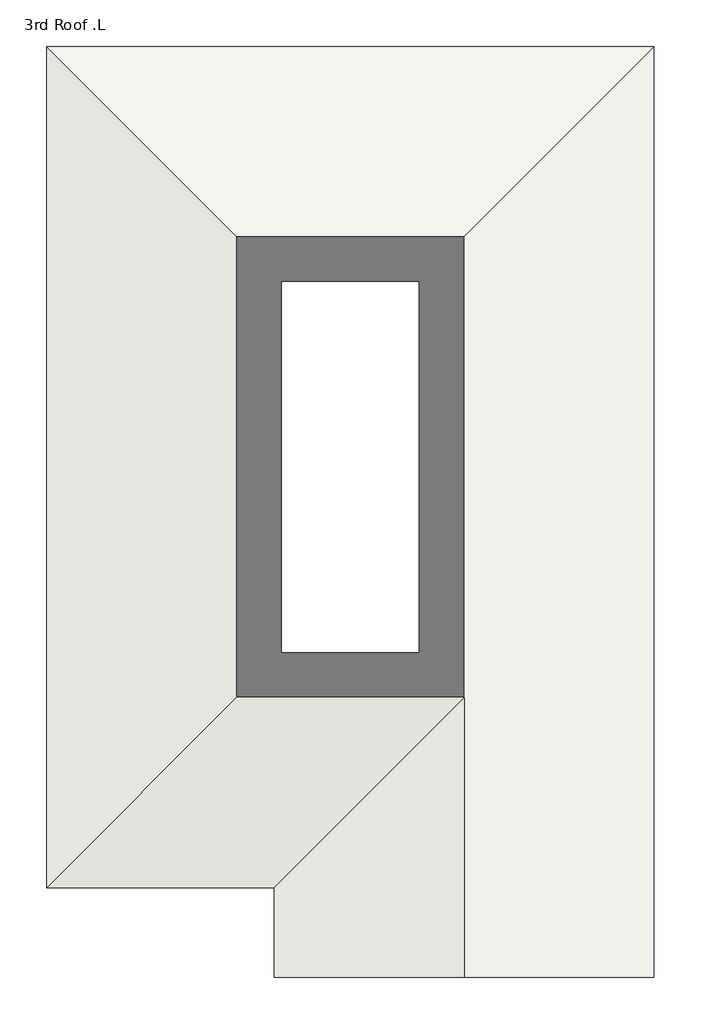
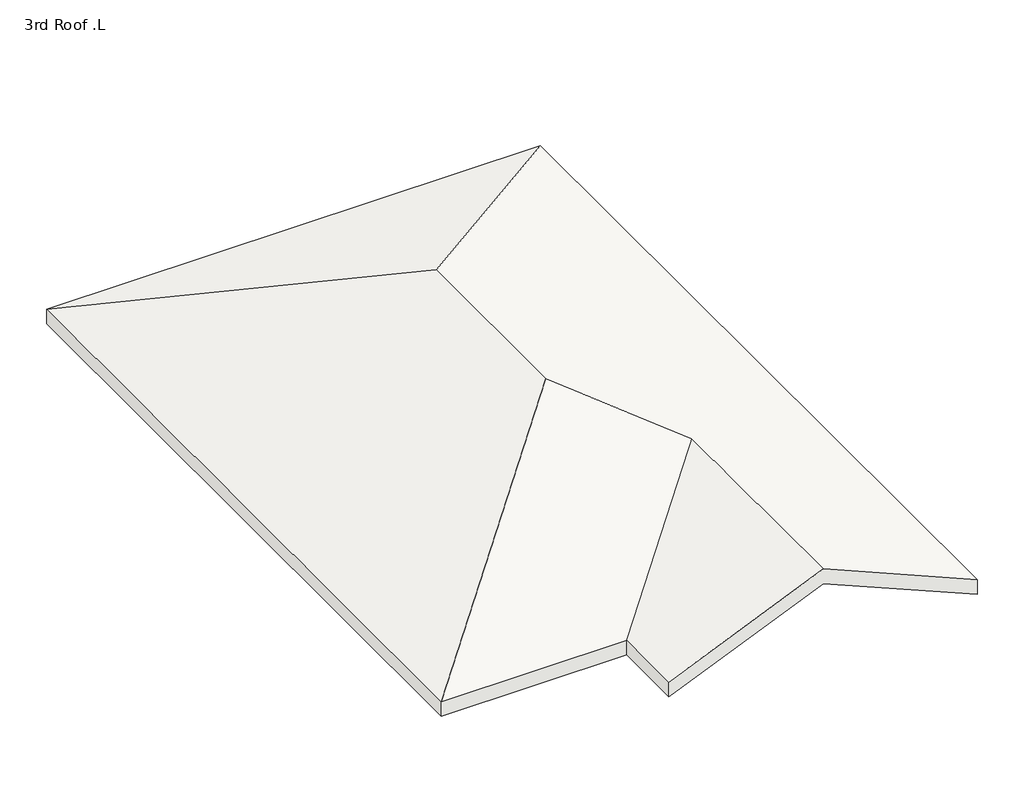
# One storey: 1 roof.
"""IFC4 building model written with IfcOpenShell, lengths in millimetres."""

from ifc_helpers import new_model, si_unit, origin, place, context, project, spatial, faceted_brep, element, save

model = new_model("IFC4")

# Units and contexts
model_context = context("Model", 3, world=origin())
ifc_project = project(units=[si_unit("LENGTHUNIT", "METRE", prefix="MILLI")], contexts=[model_context])

# Site, building, storey
site = spatial("IfcSite", under=ifc_project)
building = spatial("IfcBuilding", under=site)
storey = spatial("IfcBuildingStorey", under=building, Name="3rd Roof .L", Elevation=6400.0)

# Roof
placement = place(None, origin())
element("IfcRoof", 1, ObjectType="300mm roof", at=placement, inside=storey, context=model_context, shape_type="Brep", body=[
    faceted_brep([(3859.2341997, 8934.8567137, 5890.6302205), (-1340.7658003, 3734.8567137, 8097.8992648), (-6540.7658003, 8934.8567137, 5890.6302205), (-1340.7658003, -265.1432863, 8097.8992648), (-6540.7658003, -5465.1432863, 5890.6302205), (3859.2341997, -7003.2432863, 5890.6302205), (609.2341997, -7003.2432863, 7270.1733732), (609.2341997, -2215.1432863, 7270.1733732), (-2640.7658003, -7003.2432863, 5890.6302205), (-2640.7658003, -5465.1432863, 5890.6302205), (3859.2341997, 8934.8567137, 6216.5383338), (-6540.7658003, 8934.8567137, 6216.5383338), (-1340.7658003, 3734.8567137, 8423.8073781), (-6540.7658003, -5465.1432863, 6216.5383338), (-1340.7658003, -265.1432863, 8423.8073781), (3859.2341997, -7003.2432863, 6216.5383338), (609.2341997, -2215.1432863, 7596.0814865), (609.2341997, -7003.2432863, 7596.0814865), (-2640.7658003, -7003.2432863, 6216.5383338), (-2640.7658003, -5465.1432863, 6216.5383338)], [[[0, 1, 2]], [[2, 1, 3, 4]], [[5, 6, 7, 3, 1, 0]], [[8, 9, 7, 6]], [[9, 4, 3, 7]], [[10, 11, 12]], [[11, 13, 14, 12]], [[15, 10, 12, 14, 16, 17]], [[18, 17, 16, 19]], [[13, 19, 16, 14]], [[0, 10, 15, 5]], [[2, 11, 10, 0]], [[4, 13, 11, 2]], [[9, 19, 13, 4]], [[8, 18, 19, 9]], [[15, 17, 18, 8, 6, 5]]]),
])

save(model, "model.ifc")

# Revit data of these elements
# Type "300mm roof"
#   Assembly Code = "B1020"
# Element 1 (IfcRoof, "300mm roof")
#   built-in parameter 1001705 = 27.6372 (stored number, unit not read)
#   built-in parameter 1001701 = -1.67116 (stored number, unit not read)
#   built-in parameter 1001710 = 33615
#   Phase Created = New Construction
#   Materials on its faces: "Structure, Steel Bar Joist Layer"
# Materials
#   "Structure, Steel Bar Joist Layer": class "Metal", colour RGB 127 127 127, transparency 0, Description = "Bar joists, thermal airspace", Cost = 0
